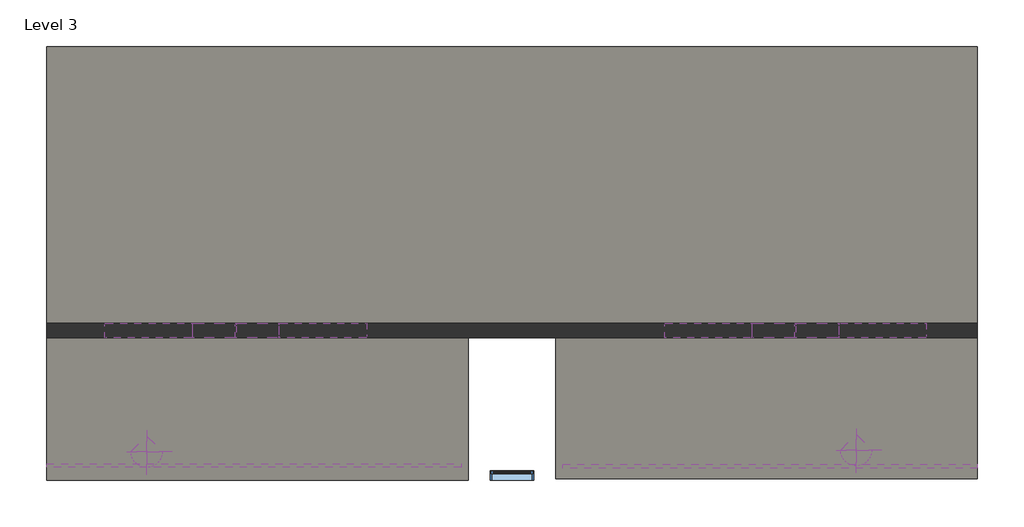
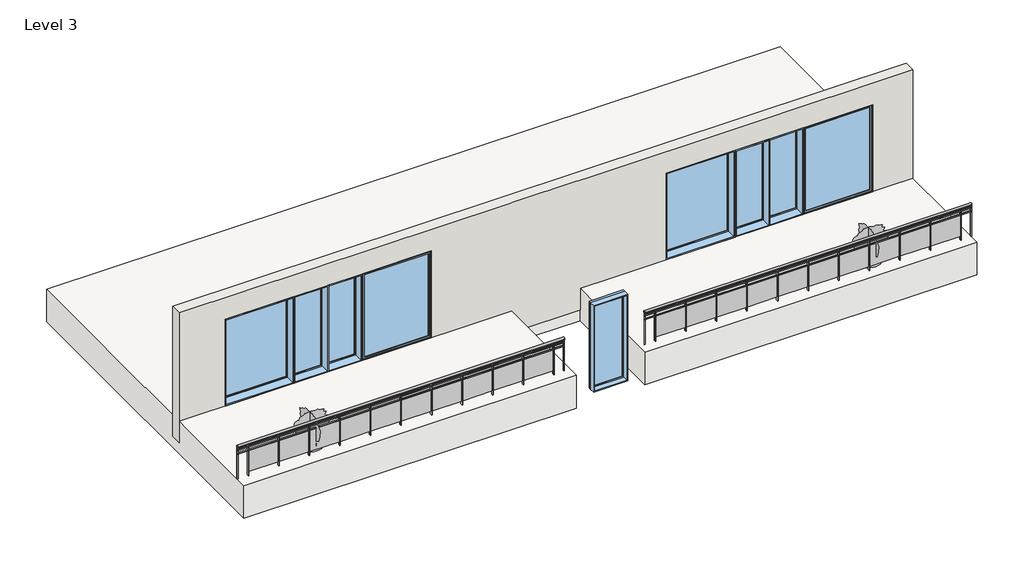
# One storey: 9 windows, 2 geographic elements, 2 railings, 1 slab, 1 wall.
"""IFC4 building model written with IfcOpenShell, lengths in millimetres."""

from ifc_helpers import new_model, si_unit, point, frame, origin, place, context, project, spatial, polyline, ellipse_curve, trimmed, outline, extrude, faceted_brep, transform, mapped, element, save
from ifc_brep_helpers import plane_surface, extruded_surface, advanced_brep
from components import geographic_element_e27c54a3, window_a209d960, window_307ff736, window_1de08d8e, window_9610881e

model = new_model("IFC4")

# Units and contexts
model_context = context("Model", 3, world=origin())
ifc_project = project(units=[si_unit("LENGTHUNIT", "METRE", prefix="MILLI")], contexts=[model_context])

# Site, building, storey
site = spatial("IfcSite", under=ifc_project)
building = spatial("IfcBuilding", under=site)
storey = spatial("IfcBuildingStorey", under=building, Name="Level 3", Elevation=6096.0)

# Geographic elements
placement = place(None, origin())
geographic_element_shape = geographic_element_e27c54a3(model_context)
element("IfcGeographicElement", 1, ObjectType="RPC Shrub : Cedar Shrub 3'-0\"", at=placement, inside=storey, context=model_context, shape_type="MappedRepresentation", body=[
    mapped(geographic_element_shape, transform((-717.5856066, 3526.7740855, 7651.75), x_axis=(1.0, 0.0, 0.0), y_axis=(0.0, 1.0, 0.0), z_axis=(0.0, 0.0, 1.0))),
])
element("IfcGeographicElement", 2, ObjectType="RPC Shrub : Cedar Shrub 3'-0\"", at=placement, inside=storey, context=model_context, shape_type="MappedRepresentation", body=[
    mapped(geographic_element_shape, transform((-15595.2031131, 3490.853061, 7702.55), x_axis=(1.0, 0.0, 0.0), y_axis=(0.0, 1.0, 0.0), z_axis=(0.0, 0.0, 1.0))),
])

# Railings
element("IfcRailing", 3, ObjectType="Glass Panel - Bottom Fill", at=placement, inside=storey, context=model_context, shape_type="SolidModel", body=[
    advanced_brep(
    [(-17688.8338476, 3238.7223265, 8534.4), (-17688.8338476, 3162.5223265, 8534.4), (-9002.0338476, 3238.7223265, 8534.4), (-9002.0338476, 3162.5223265, 8534.4)],
    [
        (0, 1, ellipse_curve(frame((-17688.8338476, 3200.6223265, 8534.4), z_axis=(-1.0, 0.0, 0.0), x_axis=(0.0, -1.0, 0.0)), 38.1, 28.575)),
        (1, 0, ellipse_curve(frame((-17688.8338476, 3200.6223265, 8534.4), z_axis=(-1.0, 0.0, 0.0), x_axis=(0.0, -1.0, 0.0)), 38.1, 28.575)),
        (2, 3, ellipse_curve(frame((-9002.0338476, 3200.6223265, 8534.4), z_axis=(1.0, 0.0, 0.0), x_axis=(0.0, -1.0, 0.0)), 38.1, 28.575)),
        (3, 2, ellipse_curve(frame((-9002.0338476, 3200.6223265, 8534.4), z_axis=(1.0, 0.0, 0.0), x_axis=(0.0, -1.0, 0.0)), 38.1, 28.575)),
        (0, 2),
        (3, 1),
    ],
    [
        plane_surface(frame((-17688.8338476, 3200.6223265, 8534.4), z_axis=(-1.0, 0.0, 0.0), x_axis=(0.0, 1.0, 0.0))),
        plane_surface(frame((-9002.0338476, 3200.6223265, 8534.4), z_axis=(1.0, 0.0, 0.0), x_axis=(0.0, 1.0, 0.0))),
        extruded_surface(trimmed(ellipse_curve(frame((-9002.0338476, 3200.6223265, 8534.4), z_axis=(-1.0, 0.0, 0.0), x_axis=(0.0, -1.0, 0.0)), 38.1, 28.575), [point((-9002.0338476, 3238.7223265, 8534.4))], [point((-9002.0338476, 3162.5223265, 8534.4))], True, "CARTESIAN"), (-8686.8, 0.0, 0.0), 8686.8),
        extruded_surface(trimmed(ellipse_curve(frame((-9002.0338476, 3200.6223265, 8534.4), z_axis=(-1.0, 0.0, 0.0), x_axis=(0.0, -1.0, 0.0)), 38.1, 28.575), [point((-9002.0338476, 3162.5223265, 8534.4))], [point((-9002.0338476, 3238.7223265, 8534.4))], True, "CARTESIAN"), (-8686.8, 0.0, 0.0), 8686.8),
    ],
    [
        (0, [[1, 2]]),
        (1, [[3, 4]]),
        (2, [[-1, 5, -4, 6]]),
        (3, [[-2, -6, -3, -5]]),
    ],
),
    extrude(outline(polyline([(-17688.8338476, 3187.9223265), (-17688.8338476, 3213.3223265), (-9002.0338476, 3213.3223265), (-9002.0338476, 3187.9223265), (-17688.8338476, 3187.9223265)])), frame((0.0, 0.0, 8420.1), z_axis=(0.0, 0.0, 1.0), x_axis=(1.0, 0.0, 0.0)), (0.0, 0.0, 1.0), 25.4),
    extrude(outline(polyline([(-17688.8338476, 3187.9223265), (-17688.8338476, 3213.3223265), (-9002.0338476, 3213.3223265), (-9002.0338476, 3187.9223265), (-17688.8338476, 3187.9223265)])), frame((0.0, 0.0, 8318.5), z_axis=(0.0, 0.0, 1.0), x_axis=(1.0, 0.0, 0.0)), (0.0, 0.0, 1.0), 25.4),
    extrude(outline(polyline([(-9287.7838476, 3175.2223265), (-9287.7838476, 3226.0223265), (-9275.0838476, 3226.0223265), (-9275.0838476, 3175.2223265), (-9287.7838476, 3175.2223265)])), frame((0.0, 0.0, 7620.0), z_axis=(0.0, 0.0, 1.0), x_axis=(1.0, 0.0, 0.0)), (0.0, 0.0, 1.0), 885.6788223),
    extrude(outline(polyline([(-10094.2338476, 3207.1574835), (-9281.4338476, 3207.1574835), (-9281.4338476, 3200.8074835), (-10094.2338476, 3200.8074835), (-10094.2338476, 3207.1574835)])), frame((0.0, 0.0, 7721.6), z_axis=(0.0, 0.0, 1.0), x_axis=(1.0, 0.0, 0.0)), (0.0, 0.0, 1.0), 596.9),
    extrude(outline(polyline([(-10100.5838476, 3175.2223265), (-10100.5838476, 3226.0223265), (-10087.8838476, 3226.0223265), (-10087.8838476, 3175.2223265), (-10100.5838476, 3175.2223265)])), frame((0.0, 0.0, 7620.0), z_axis=(0.0, 0.0, 1.0), x_axis=(1.0, 0.0, 0.0)), (0.0, 0.0, 1.0), 885.6788223),
    extrude(outline(polyline([(-10907.0338476, 3207.1574835), (-10094.2338476, 3207.1574835), (-10094.2338476, 3200.8074835), (-10907.0338476, 3200.8074835), (-10907.0338476, 3207.1574835)])), frame((0.0, 0.0, 7721.6), z_axis=(0.0, 0.0, 1.0), x_axis=(1.0, 0.0, 0.0)), (0.0, 0.0, 1.0), 596.9),
    extrude(outline(polyline([(-10913.3838476, 3175.2223265), (-10913.3838476, 3226.0223265), (-10900.6838476, 3226.0223265), (-10900.6838476, 3175.2223265), (-10913.3838476, 3175.2223265)])), frame((0.0, 0.0, 7620.0), z_axis=(0.0, 0.0, 1.0), x_axis=(1.0, 0.0, 0.0)), (0.0, 0.0, 1.0), 885.6788223),
    extrude(outline(polyline([(-11719.8338476, 3207.1574835), (-10907.0338476, 3207.1574835), (-10907.0338476, 3200.8074835), (-11719.8338476, 3200.8074835), (-11719.8338476, 3207.1574835)])), frame((0.0, 0.0, 7721.6), z_axis=(0.0, 0.0, 1.0), x_axis=(1.0, 0.0, 0.0)), (0.0, 0.0, 1.0), 596.9),
    extrude(outline(polyline([(-11726.1838476, 3175.2223265), (-11726.1838476, 3226.0223265), (-11713.4838476, 3226.0223265), (-11713.4838476, 3175.2223265), (-11726.1838476, 3175.2223265)])), frame((0.0, 0.0, 7620.0), z_axis=(0.0, 0.0, 1.0), x_axis=(1.0, 0.0, 0.0)), (0.0, 0.0, 1.0), 885.6788223),
    extrude(outline(polyline([(-12532.6338476, 3207.1574835), (-11719.8338476, 3207.1574835), (-11719.8338476, 3200.8074835), (-12532.6338476, 3200.8074835), (-12532.6338476, 3207.1574835)])), frame((0.0, 0.0, 7721.6), z_axis=(0.0, 0.0, 1.0), x_axis=(1.0, 0.0, 0.0)), (0.0, 0.0, 1.0), 596.9),
    extrude(outline(polyline([(-12538.9838476, 3175.2223265), (-12538.9838476, 3226.0223265), (-12526.2838476, 3226.0223265), (-12526.2838476, 3175.2223265), (-12538.9838476, 3175.2223265)])), frame((0.0, 0.0, 7620.0), z_axis=(0.0, 0.0, 1.0), x_axis=(1.0, 0.0, 0.0)), (0.0, 0.0, 1.0), 885.6788223),
    extrude(outline(polyline([(-13345.4338476, 3207.1574835), (-12532.6338476, 3207.1574835), (-12532.6338476, 3200.8074835), (-13345.4338476, 3200.8074835), (-13345.4338476, 3207.1574835)])), frame((0.0, 0.0, 7721.6), z_axis=(0.0, 0.0, 1.0), x_axis=(1.0, 0.0, 0.0)), (0.0, 0.0, 1.0), 596.9),
    extrude(outline(polyline([(-13351.7838476, 3175.2223265), (-13351.7838476, 3226.0223265), (-13339.0838476, 3226.0223265), (-13339.0838476, 3175.2223265), (-13351.7838476, 3175.2223265)])), frame((0.0, 0.0, 7620.0), z_axis=(0.0, 0.0, 1.0), x_axis=(1.0, 0.0, 0.0)), (0.0, 0.0, 1.0), 885.6788223),
    extrude(outline(polyline([(-14158.2338476, 3207.1574835), (-13345.4338476, 3207.1574835), (-13345.4338476, 3200.8074835), (-14158.2338476, 3200.8074835), (-14158.2338476, 3207.1574835)])), frame((0.0, 0.0, 7721.6), z_axis=(0.0, 0.0, 1.0), x_axis=(1.0, 0.0, 0.0)), (0.0, 0.0, 1.0), 596.9),
    extrude(outline(polyline([(-14164.5838476, 3175.2223265), (-14164.5838476, 3226.0223265), (-14151.8838476, 3226.0223265), (-14151.8838476, 3175.2223265), (-14164.5838476, 3175.2223265)])), frame((0.0, 0.0, 7620.0), z_axis=(0.0, 0.0, 1.0), x_axis=(1.0, 0.0, 0.0)), (0.0, 0.0, 1.0), 885.6788223),
    extrude(outline(polyline([(-14971.0338476, 3207.1574835), (-14158.2338476, 3207.1574835), (-14158.2338476, 3200.8074835), (-14971.0338476, 3200.8074835), (-14971.0338476, 3207.1574835)])), frame((0.0, 0.0, 7721.6), z_axis=(0.0, 0.0, 1.0), x_axis=(1.0, 0.0, 0.0)), (0.0, 0.0, 1.0), 596.9),
    extrude(outline(polyline([(-14977.3838476, 3175.2223265), (-14977.3838476, 3226.0223265), (-14964.6838476, 3226.0223265), (-14964.6838476, 3175.2223265), (-14977.3838476, 3175.2223265)])), frame((0.0, 0.0, 7620.0), z_axis=(0.0, 0.0, 1.0), x_axis=(1.0, 0.0, 0.0)), (0.0, 0.0, 1.0), 885.6788223),
    extrude(outline(polyline([(-15783.8338476, 3207.1574835), (-14971.0338476, 3207.1574835), (-14971.0338476, 3200.8074835), (-15783.8338476, 3200.8074835), (-15783.8338476, 3207.1574835)])), frame((0.0, 0.0, 7721.6), z_axis=(0.0, 0.0, 1.0), x_axis=(1.0, 0.0, 0.0)), (0.0, 0.0, 1.0), 596.9),
    extrude(outline(polyline([(-15790.1838476, 3175.2223265), (-15790.1838476, 3226.0223265), (-15777.4838476, 3226.0223265), (-15777.4838476, 3175.2223265), (-15790.1838476, 3175.2223265)])), frame((0.0, 0.0, 7620.0), z_axis=(0.0, 0.0, 1.0), x_axis=(1.0, 0.0, 0.0)), (0.0, 0.0, 1.0), 885.6788223),
    extrude(outline(polyline([(-16596.6338476, 3207.1574835), (-15783.8338476, 3207.1574835), (-15783.8338476, 3200.8074835), (-16596.6338476, 3200.8074835), (-16596.6338476, 3207.1574835)])), frame((0.0, 0.0, 7721.6), z_axis=(0.0, 0.0, 1.0), x_axis=(1.0, 0.0, 0.0)), (0.0, 0.0, 1.0), 596.9),
    extrude(outline(polyline([(-16602.9838476, 3175.2223265), (-16602.9838476, 3226.0223265), (-16590.2838476, 3226.0223265), (-16590.2838476, 3175.2223265), (-16602.9838476, 3175.2223265)])), frame((0.0, 0.0, 7620.0), z_axis=(0.0, 0.0, 1.0), x_axis=(1.0, 0.0, 0.0)), (0.0, 0.0, 1.0), 885.6788223),
    extrude(outline(polyline([(-17409.4338476, 3207.1574835), (-16596.6338476, 3207.1574835), (-16596.6338476, 3200.8074835), (-17409.4338476, 3200.8074835), (-17409.4338476, 3207.1574835)])), frame((0.0, 0.0, 7721.6), z_axis=(0.0, 0.0, 1.0), x_axis=(1.0, 0.0, 0.0)), (0.0, 0.0, 1.0), 596.9),
    extrude(outline(polyline([(-17415.7838476, 3175.2223265), (-17415.7838476, 3226.0223265), (-17403.0838476, 3226.0223265), (-17403.0838476, 3175.2223265), (-17415.7838476, 3175.2223265)])), frame((0.0, 0.0, 7620.0), z_axis=(0.0, 0.0, 1.0), x_axis=(1.0, 0.0, 0.0)), (0.0, 0.0, 1.0), 885.6788223),
    extrude(outline(polyline([(-9014.7338476, 3191.0973265), (-9014.7338476, 3210.1473265), (-8995.6838476, 3210.1473265), (-8995.6838476, 3191.0973265), (-9014.7338476, 3191.0973265)])), frame((0.0, 0.0, 7620.0), z_axis=(0.0, 0.0, 1.0), x_axis=(1.0, 0.0, 0.0)), (0.0, 0.0, 1.0), 885.6788223),
    extrude(outline(polyline([(-17695.1838476, 3191.0973265), (-17695.1838476, 3210.1473265), (-17676.1338476, 3210.1473265), (-17676.1338476, 3191.0973265), (-17695.1838476, 3191.0973265)])), frame((0.0, 0.0, 7620.0), z_axis=(0.0, 0.0, 1.0), x_axis=(1.0, 0.0, 0.0)), (0.0, 0.0, 1.0), 885.6788223),
])
element("IfcRailing", 4, ObjectType="Glass Panel - Bottom Fill", at=placement, inside=storey, context=model_context, shape_type="SolidModel", body=[
    advanced_brep(
    [(-6868.4338476, 3226.0223265, 8534.4), (-6868.4338476, 3149.8223265, 8534.4), (1818.3661524, 3226.0223265, 8534.4), (1818.3661524, 3149.8223265, 8534.4)],
    [
        (0, 1, ellipse_curve(frame((-6868.4338476, 3187.9223265, 8534.4), z_axis=(-1.0, 0.0, 0.0), x_axis=(0.0, -1.0, 0.0)), 38.1, 28.575)),
        (1, 0, ellipse_curve(frame((-6868.4338476, 3187.9223265, 8534.4), z_axis=(-1.0, 0.0, 0.0), x_axis=(0.0, -1.0, 0.0)), 38.1, 28.575)),
        (2, 3, ellipse_curve(frame((1818.3661524, 3187.9223265, 8534.4), z_axis=(1.0, 0.0, 0.0), x_axis=(0.0, -1.0, 0.0)), 38.1, 28.575)),
        (3, 2, ellipse_curve(frame((1818.3661524, 3187.9223265, 8534.4), z_axis=(1.0, 0.0, 0.0), x_axis=(0.0, -1.0, 0.0)), 38.1, 28.575)),
        (0, 2),
        (3, 1),
    ],
    [
        plane_surface(frame((-6868.4338476, 3187.9223265, 8534.4), z_axis=(-1.0, 0.0, 0.0), x_axis=(0.0, 1.0, 0.0))),
        plane_surface(frame((1818.3661524, 3187.9223265, 8534.4), z_axis=(1.0, 0.0, 0.0), x_axis=(0.0, 1.0, 0.0))),
        extruded_surface(trimmed(ellipse_curve(frame((1818.3661524, 3187.9223265, 8534.4), z_axis=(-1.0, 0.0, 0.0), x_axis=(0.0, -1.0, 0.0)), 38.1, 28.575), [point((1818.3661524, 3226.0223265, 8534.4))], [point((1818.3661524, 3149.8223265, 8534.4))], True, "CARTESIAN"), (-8686.8, 0.0, 0.0), 8686.8),
        extruded_surface(trimmed(ellipse_curve(frame((1818.3661524, 3187.9223265, 8534.4), z_axis=(-1.0, 0.0, 0.0), x_axis=(0.0, -1.0, 0.0)), 38.1, 28.575), [point((1818.3661524, 3149.8223265, 8534.4))], [point((1818.3661524, 3226.0223265, 8534.4))], True, "CARTESIAN"), (-8686.8, 0.0, 0.0), 8686.8),
    ],
    [
        (0, [[1, 2]]),
        (1, [[3, 4]]),
        (2, [[-1, 5, -4, 6]]),
        (3, [[-2, -6, -3, -5]]),
    ],
),
    extrude(outline(polyline([(-6868.4338476, 3175.2223265), (-6868.4338476, 3200.6223265), (1818.3661524, 3200.6223265), (1818.3661524, 3175.2223265), (-6868.4338476, 3175.2223265)])), frame((0.0, 0.0, 8420.1), z_axis=(0.0, 0.0, 1.0), x_axis=(1.0, 0.0, 0.0)), (0.0, 0.0, 1.0), 25.4),
    extrude(outline(polyline([(-6868.4338476, 3175.2223265), (-6868.4338476, 3200.6223265), (1818.3661524, 3200.6223265), (1818.3661524, 3175.2223265), (-6868.4338476, 3175.2223265)])), frame((0.0, 0.0, 8318.5), z_axis=(0.0, 0.0, 1.0), x_axis=(1.0, 0.0, 0.0)), (0.0, 0.0, 1.0), 25.4),
    extrude(outline(polyline([(1532.6161524, 3162.5223265), (1532.6161524, 3213.3223265), (1545.3161524, 3213.3223265), (1545.3161524, 3162.5223265), (1532.6161524, 3162.5223265)])), frame((0.0, 0.0, 7620.0), z_axis=(0.0, 0.0, 1.0), x_axis=(1.0, 0.0, 0.0)), (0.0, 0.0, 1.0), 885.6788223),
    extrude(outline(polyline([(726.1661524, 3194.4574835), (1538.9661524, 3194.4574835), (1538.9661524, 3188.1074835), (726.1661524, 3188.1074835), (726.1661524, 3194.4574835)])), frame((0.0, 0.0, 7721.6), z_axis=(0.0, 0.0, 1.0), x_axis=(1.0, 0.0, 0.0)), (0.0, 0.0, 1.0), 596.9),
    extrude(outline(polyline([(719.8161524, 3162.5223265), (719.8161524, 3213.3223265), (732.5161524, 3213.3223265), (732.5161524, 3162.5223265), (719.8161524, 3162.5223265)])), frame((0.0, 0.0, 7620.0), z_axis=(0.0, 0.0, 1.0), x_axis=(1.0, 0.0, 0.0)), (0.0, 0.0, 1.0), 885.6788223),
    extrude(outline(polyline([(-86.6338476, 3194.4574835), (726.1661524, 3194.4574835), (726.1661524, 3188.1074835), (-86.6338476, 3188.1074835), (-86.6338476, 3194.4574835)])), frame((0.0, 0.0, 7721.6), z_axis=(0.0, 0.0, 1.0), x_axis=(1.0, 0.0, 0.0)), (0.0, 0.0, 1.0), 596.9),
    extrude(outline(polyline([(-92.9838476, 3162.5223265), (-92.9838476, 3213.3223265), (-80.2838476, 3213.3223265), (-80.2838476, 3162.5223265), (-92.9838476, 3162.5223265)])), frame((0.0, 0.0, 7620.0), z_axis=(0.0, 0.0, 1.0), x_axis=(1.0, 0.0, 0.0)), (0.0, 0.0, 1.0), 885.6788223),
    extrude(outline(polyline([(-899.4338476, 3194.4574835), (-86.6338476, 3194.4574835), (-86.6338476, 3188.1074835), (-899.4338476, 3188.1074835), (-899.4338476, 3194.4574835)])), frame((0.0, 0.0, 7721.6), z_axis=(0.0, 0.0, 1.0), x_axis=(1.0, 0.0, 0.0)), (0.0, 0.0, 1.0), 596.9),
    extrude(outline(polyline([(-905.7838476, 3162.5223265), (-905.7838476, 3213.3223265), (-893.0838476, 3213.3223265), (-893.0838476, 3162.5223265), (-905.7838476, 3162.5223265)])), frame((0.0, 0.0, 7620.0), z_axis=(0.0, 0.0, 1.0), x_axis=(1.0, 0.0, 0.0)), (0.0, 0.0, 1.0), 885.6788223),
    extrude(outline(polyline([(-1712.2338476, 3194.4574835), (-899.4338476, 3194.4574835), (-899.4338476, 3188.1074835), (-1712.2338476, 3188.1074835), (-1712.2338476, 3194.4574835)])), frame((0.0, 0.0, 7721.6), z_axis=(0.0, 0.0, 1.0), x_axis=(1.0, 0.0, 0.0)), (0.0, 0.0, 1.0), 596.9),
    extrude(outline(polyline([(-1718.5838476, 3162.5223265), (-1718.5838476, 3213.3223265), (-1705.8838476, 3213.3223265), (-1705.8838476, 3162.5223265), (-1718.5838476, 3162.5223265)])), frame((0.0, 0.0, 7620.0), z_axis=(0.0, 0.0, 1.0), x_axis=(1.0, 0.0, 0.0)), (0.0, 0.0, 1.0), 885.6788223),
    extrude(outline(polyline([(-2525.0338476, 3194.4574835), (-1712.2338476, 3194.4574835), (-1712.2338476, 3188.1074835), (-2525.0338476, 3188.1074835), (-2525.0338476, 3194.4574835)])), frame((0.0, 0.0, 7721.6), z_axis=(0.0, 0.0, 1.0), x_axis=(1.0, 0.0, 0.0)), (0.0, 0.0, 1.0), 596.9),
    extrude(outline(polyline([(-2531.3838476, 3162.5223265), (-2531.3838476, 3213.3223265), (-2518.6838476, 3213.3223265), (-2518.6838476, 3162.5223265), (-2531.3838476, 3162.5223265)])), frame((0.0, 0.0, 7620.0), z_axis=(0.0, 0.0, 1.0), x_axis=(1.0, 0.0, 0.0)), (0.0, 0.0, 1.0), 885.6788223),
    extrude(outline(polyline([(-3337.8338476, 3194.4574835), (-2525.0338476, 3194.4574835), (-2525.0338476, 3188.1074835), (-3337.8338476, 3188.1074835), (-3337.8338476, 3194.4574835)])), frame((0.0, 0.0, 7721.6), z_axis=(0.0, 0.0, 1.0), x_axis=(1.0, 0.0, 0.0)), (0.0, 0.0, 1.0), 596.9),
    extrude(outline(polyline([(-3344.1838476, 3162.5223265), (-3344.1838476, 3213.3223265), (-3331.4838476, 3213.3223265), (-3331.4838476, 3162.5223265), (-3344.1838476, 3162.5223265)])), frame((0.0, 0.0, 7620.0), z_axis=(0.0, 0.0, 1.0), x_axis=(1.0, 0.0, 0.0)), (0.0, 0.0, 1.0), 885.6788223),
    extrude(outline(polyline([(-4150.6338476, 3194.4574835), (-3337.8338476, 3194.4574835), (-3337.8338476, 3188.1074835), (-4150.6338476, 3188.1074835), (-4150.6338476, 3194.4574835)])), frame((0.0, 0.0, 7721.6), z_axis=(0.0, 0.0, 1.0), x_axis=(1.0, 0.0, 0.0)), (0.0, 0.0, 1.0), 596.9),
    extrude(outline(polyline([(-4156.9838476, 3162.5223265), (-4156.9838476, 3213.3223265), (-4144.2838476, 3213.3223265), (-4144.2838476, 3162.5223265), (-4156.9838476, 3162.5223265)])), frame((0.0, 0.0, 7620.0), z_axis=(0.0, 0.0, 1.0), x_axis=(1.0, 0.0, 0.0)), (0.0, 0.0, 1.0), 885.6788223),
    extrude(outline(polyline([(-4963.4338476, 3194.4574835), (-4150.6338476, 3194.4574835), (-4150.6338476, 3188.1074835), (-4963.4338476, 3188.1074835), (-4963.4338476, 3194.4574835)])), frame((0.0, 0.0, 7721.6), z_axis=(0.0, 0.0, 1.0), x_axis=(1.0, 0.0, 0.0)), (0.0, 0.0, 1.0), 596.9),
    extrude(outline(polyline([(-4969.7838476, 3162.5223265), (-4969.7838476, 3213.3223265), (-4957.0838476, 3213.3223265), (-4957.0838476, 3162.5223265), (-4969.7838476, 3162.5223265)])), frame((0.0, 0.0, 7620.0), z_axis=(0.0, 0.0, 1.0), x_axis=(1.0, 0.0, 0.0)), (0.0, 0.0, 1.0), 885.6788223),
    extrude(outline(polyline([(-5776.2338476, 3194.4574835), (-4963.4338476, 3194.4574835), (-4963.4338476, 3188.1074835), (-5776.2338476, 3188.1074835), (-5776.2338476, 3194.4574835)])), frame((0.0, 0.0, 7721.6), z_axis=(0.0, 0.0, 1.0), x_axis=(1.0, 0.0, 0.0)), (0.0, 0.0, 1.0), 596.9),
    extrude(outline(polyline([(-5782.5838476, 3162.5223265), (-5782.5838476, 3213.3223265), (-5769.8838476, 3213.3223265), (-5769.8838476, 3162.5223265), (-5782.5838476, 3162.5223265)])), frame((0.0, 0.0, 7620.0), z_axis=(0.0, 0.0, 1.0), x_axis=(1.0, 0.0, 0.0)), (0.0, 0.0, 1.0), 885.6788223),
    extrude(outline(polyline([(-6589.0338476, 3194.4574835), (-5776.2338476, 3194.4574835), (-5776.2338476, 3188.1074835), (-6589.0338476, 3188.1074835), (-6589.0338476, 3194.4574835)])), frame((0.0, 0.0, 7721.6), z_axis=(0.0, 0.0, 1.0), x_axis=(1.0, 0.0, 0.0)), (0.0, 0.0, 1.0), 596.9),
    extrude(outline(polyline([(-6595.3838476, 3162.5223265), (-6595.3838476, 3213.3223265), (-6582.6838476, 3213.3223265), (-6582.6838476, 3162.5223265), (-6595.3838476, 3162.5223265)])), frame((0.0, 0.0, 7620.0), z_axis=(0.0, 0.0, 1.0), x_axis=(1.0, 0.0, 0.0)), (0.0, 0.0, 1.0), 885.6788223),
    extrude(outline(polyline([(1805.6661524, 3178.3973265), (1805.6661524, 3197.4473265), (1824.7161524, 3197.4473265), (1824.7161524, 3178.3973265), (1805.6661524, 3178.3973265)])), frame((0.0, 0.0, 7620.0), z_axis=(0.0, 0.0, 1.0), x_axis=(1.0, 0.0, 0.0)), (0.0, 0.0, 1.0), 885.6788223),
    extrude(outline(polyline([(-6874.7838476, 3178.3973265), (-6874.7838476, 3197.4473265), (-6855.7338476, 3197.4473265), (-6855.7338476, 3178.3973265), (-6874.7838476, 3178.3973265)])), frame((0.0, 0.0, 7620.0), z_axis=(0.0, 0.0, 1.0), x_axis=(1.0, 0.0, 0.0)), (0.0, 0.0, 1.0), 885.6788223),
])

# Slab
element("IfcSlab", 5, ObjectType="Generic - 3'", at=placement, inside=storey, context=model_context, shape_type="SweptSolid", body=[
    extrude(outline(polyline([(1818.3661524, 11989.0223265), (1818.3661524, 2921.2223265), (-7020.8338476, 2921.2223265), (-7020.8338476, 5893.0223265), (-8849.6338476, 5893.0223265), (-8849.6338476, 2895.8223265), (-17688.8338476, 2895.8223265), (-17688.8338476, 11989.0223265), (1818.3661524, 11989.0223265)])), frame((0.0, 0.0, 6705.6), z_axis=(0.0, 0.0, 1.0), x_axis=(1.0, 0.0, 0.0)), (0.0, 0.0, 1.0), 914.4),
])

# Wall
element("IfcWall", 6, ObjectType="Generic - 12\" black", at=placement, inside=storey, context=model_context, shape_type="Brep", body=[
    faceted_brep([(-17688.8338476, 5880.3223265, 7010.4), (1818.3661524, 5880.3223265, 7010.4), (1818.3661524, 5880.3223265, 10668.0), (-6868.4338476, 5880.3223265, 10668.0), (-7173.2338476, 5880.3223265, 10668.0), (-8697.2338476, 5880.3223265, 10668.0), (-9002.0338476, 5880.3223265, 10668.0), (-17688.8338476, 5880.3223265, 10668.0), (751.5661524, 5880.3223265, 10058.4), (751.5661524, 5880.3223265, 7620.0), (-1077.2338476, 5880.3223265, 7620.0), (-1077.2338476, 5880.3223265, 10058.4), (-1086.7588476, 5880.3223265, 10052.683689), (-1086.7588476, 5880.3223265, 7614.283689), (-2896.5088476, 5880.3223265, 7614.283689), (-2896.5088476, 5880.3223265, 10052.683689), (-2906.0338476, 5880.3223265, 10058.4), (-2906.0338476, 5880.3223265, 7620.0), (-4734.8338476, 5880.3223265, 7620.0), (-4734.8338476, 5880.3223265, 10058.4), (-10983.2338476, 5880.3223265, 10058.4), (-10983.2338476, 5880.3223265, 7620.0), (-12812.0338476, 5880.3223265, 7620.0), (-12812.0338476, 5880.3223265, 10058.4), (-14631.3088476, 5880.3223265, 10052.683689), (-12821.5588476, 5880.3223265, 10052.683689), (-12821.5588476, 5880.3223265, 7614.283689), (-14631.3088476, 5880.3223265, 7614.283689), (-14640.8338476, 5880.3223265, 10058.4), (-14640.8338476, 5880.3223265, 7620.0), (-16469.6338476, 5880.3223265, 7620.0), (-16469.6338476, 5880.3223265, 10058.4), (1818.3661524, 6185.1223265, 7010.4), (-17688.8338476, 6185.1223265, 7010.4), (-17688.8338476, 6185.1223265, 10668.0), (1818.3661524, 6185.1223265, 10668.0), (751.5661524, 6185.1223265, 10058.4), (-1077.2338476, 6185.1223265, 10058.4), (-1077.2338476, 6185.1223265, 7620.0), (751.5661524, 6185.1223265, 7620.0), (-1086.7588476, 6185.1223265, 7614.283689), (-1086.7588476, 6185.1223265, 10052.683689), (-2896.5088476, 6185.1223265, 10052.683689), (-2896.5088476, 6185.1223265, 7614.283689), (-2906.0338476, 6185.1223265, 10058.4), (-4734.8338476, 6185.1223265, 10058.4), (-4734.8338476, 6185.1223265, 7620.0), (-2906.0338476, 6185.1223265, 7620.0), (-10983.2338476, 6185.1223265, 10058.4), (-12812.0338476, 6185.1223265, 10058.4), (-12812.0338476, 6185.1223265, 7620.0), (-10983.2338476, 6185.1223265, 7620.0), (-14631.3088476, 6185.1223265, 7614.283689), (-12821.5588476, 6185.1223265, 7614.283689), (-12821.5588476, 6185.1223265, 10052.683689), (-14631.3088476, 6185.1223265, 10052.683689), (-14640.8338476, 6185.1223265, 10058.4), (-16469.6338476, 6185.1223265, 10058.4), (-16469.6338476, 6185.1223265, 7620.0), (-14640.8338476, 6185.1223265, 7620.0)], [[[0, 1, 2, 3, 4, 5, 6, 7], [8, 9, 10, 11], [12, 13, 14, 15], [16, 17, 18, 19], [20, 21, 22, 23], [24, 25, 26, 27], [28, 29, 30, 31]], [[32, 33, 34, 35], [36, 37, 38, 39], [40, 41, 42, 43], [44, 45, 46, 47], [48, 49, 50, 51], [52, 53, 54, 55], [56, 57, 58, 59]], [[1, 0, 33, 32]], [[7, 6, 5, 4, 3, 2, 35, 34]], [[0, 7, 34, 33]], [[2, 1, 32, 35]], [[9, 8, 36, 39]], [[10, 9, 39, 38]], [[11, 10, 38, 37]], [[8, 11, 37, 36]], [[13, 12, 41, 40]], [[13, 40, 43, 14]], [[41, 12, 15, 42]], [[14, 43, 42, 15]], [[17, 16, 44, 47]], [[18, 17, 47, 46]], [[19, 18, 46, 45]], [[16, 19, 45, 44]], [[21, 20, 48, 51]], [[22, 21, 51, 50]], [[23, 22, 50, 49]], [[20, 23, 49, 48]], [[26, 25, 54, 53]], [[26, 53, 52, 27]], [[54, 25, 24, 55]], [[27, 52, 55, 24]], [[29, 28, 56, 59]], [[30, 29, 59, 58]], [[31, 30, 58, 57]], [[28, 31, 57, 56]]]),
])

# Windows
window_shape = window_a209d960(model_context)
element("IfcWindow", 7, ObjectType="Fixed : 36\" x 96\"", at=placement, inside=storey, context=model_context, shape_type="MappedRepresentation", body=[
    mapped(window_shape, transform((-2401.2088476, 6032.7223265, 7309.483689), x_axis=(1.0, 0.0, 0.0), y_axis=(0.0, 1.0, 0.0), z_axis=(0.0, 0.0, 1.0))),
])
element("IfcWindow", 8, ObjectType="Fixed : 36\" x 96\"", at=placement, inside=storey, context=model_context, shape_type="MappedRepresentation", body=[
    mapped(window_shape, transform((-1505.8588476, 6032.7223265, 7309.483689), x_axis=(1.0, 0.0, 0.0), y_axis=(0.0, 1.0, 0.0), z_axis=(0.0, 0.0, 1.0))),
])
element("IfcWindow", 9, ObjectType="Fixed : 36\" x 96\"", at=placement, inside=storey, context=model_context, shape_type="MappedRepresentation", body=[
    mapped(window_shape, transform((-14136.0088476, 6032.7223265, 7309.483689), x_axis=(1.0, 0.0, 0.0), y_axis=(0.0, 1.0, 0.0), z_axis=(0.0, 0.0, 1.0))),
])
element("IfcWindow", 10, ObjectType="Fixed : 36\" x 96\"", at=placement, inside=storey, context=model_context, shape_type="MappedRepresentation", body=[
    mapped(window_shape, transform((-13240.6588476, 6032.7223265, 7309.483689), x_axis=(1.0, 0.0, 0.0), y_axis=(0.0, 1.0, 0.0), z_axis=(0.0, 0.0, 1.0))),
])
window_2_shape = window_307ff736(model_context)
element("IfcWindow", 11, ObjectType="Fixed : 36\" x 96\"", at=placement, inside=storey, context=model_context, shape_type="MappedRepresentation", body=[
    mapped(window_2_shape, transform((-7897.1338476, 2997.4223265, 6683.6097194), x_axis=(1.0, 0.0, 0.0), y_axis=(0.0, 1.0, 0.0), z_axis=(0.0, 0.0, 1.0))),
])
window_3_shape = window_1de08d8e(model_context)
element("IfcWindow", 12, ObjectType="Fixed : 72\" x 96\"", at=placement, inside=storey, context=model_context, shape_type="MappedRepresentation", body=[
    mapped(window_3_shape, transform((-3782.3338476, 6032.7223265, 7315.2), x_axis=(1.0, 0.0, 0.0), y_axis=(0.0, 1.0, 0.0), z_axis=(0.0, 0.0, 1.0))),
])
element("IfcWindow", 13, ObjectType="Fixed : 72\" x 96\"", at=placement, inside=storey, context=model_context, shape_type="MappedRepresentation", body=[
    mapped(window_3_shape, transform((-15517.1338476, 6032.7223265, 7315.2), x_axis=(1.0, 0.0, 0.0), y_axis=(0.0, 1.0, 0.0), z_axis=(0.0, 0.0, 1.0))),
])
window_4_shape = window_9610881e(model_context)
element("IfcWindow", 14, ObjectType="Fixed : 72\" x 96\"", at=placement, inside=storey, context=model_context, shape_type="MappedRepresentation", body=[
    mapped(window_4_shape, transform((-124.7338476, 6032.7223265, 7315.2), x_axis=(1.0, 0.0, 0.0), y_axis=(0.0, 1.0, 0.0), z_axis=(0.0, 0.0, 1.0))),
])
element("IfcWindow", 15, ObjectType="Fixed : 72\" x 96\"", at=placement, inside=storey, context=model_context, shape_type="MappedRepresentation", body=[
    mapped(window_4_shape, transform((-11859.5338476, 6032.7223265, 7315.2), x_axis=(1.0, 0.0, 0.0), y_axis=(0.0, 1.0, 0.0), z_axis=(0.0, 0.0, 1.0))),
])

save(model, "model.ifc")

# Revit data of these elements
# Type "RPC Shrub : Cedar Shrub 3'-0\""
#   Type Comments = "Cedar Shrub"
#   built-in parameter 1005198 = "{2, 15},{39, RPC-16-FUMD-ULXX-U7X6-J000-ST1L-LVER-AU},{1, 0},{1, 0},{2, 13},{1, 8},{5, Color},{1, 0},{1, 0},{3, 0.8},{3, 0.8},{3, 0.8},{1, 8},{7, BBoxMin},{1, 0},{1, 0},{1, 0},{1, 0},{1, 0},{1, 8},{7, BBoxMax},{1, 0},{1, 0},{1, 0},{1, 0},{1, 0},{2, 11},{9, RPCTypeId},{1, 0},{1, 0},{39, RPC-16-FUMD-ULXX-U7X6-J000-ST1L-LVER-AU},{1, 6},{14, RPCPlantHeight},{1, 0},{1, 0},{1, 3},{2, 11},{7, keyword},{1, 0},{1, 0},{35, :RPCs:Shrubs [General]:Geometry:RPC},{2, 11},{8, category},{1, 0},{1, 0},{16, Shrubs [General]},{2, 11},{12, LocalizedUID},{1, 0},{1, 0},{11, Cedar Shrub},{2, 14},{6, Height},{1, 0},{1, 0},{1, 3},{1, 2},{16, Cast Reflections},{1, 0},{1, 0},{1, 0},{1, 2},{12, Cast Shadows},{1, 0},{1, 0},{1, 1},{1, 2},{9, Lock View},{1, 0},{1, 0},{1, 0},{1, 4},{5, ViewC},{1, 0},{1, 0},{1, 0},{21, assetlibrary_base.fbx},{1, 5},"
#   built-in parameter 1005195 = "RPC-16-FUMD-ULXX-U7X6-J000-ST1L-LVER-AU"
#   Assembly Code = "G2050500"
#   Height = 3' - 0"
#   Default Elevation = 0
# Type "Glass Panel - Bottom Fill"
#   Assembly Code = "C2010400"
#   built-in parameter 1008612 = 0.0416667 (stored number, unit not read)
#   built-in parameter 1008611 = 0.0416667 (stored number, unit not read)
#   built-in parameter 1008609 = 0.333333 (stored number, unit not read)
#   built-in parameter 1008604 = 0.166667 (stored number, unit not read)
#   built-in parameter 1008603 = 0.166667 (stored number, unit not read)
#   Railing Height = 3' - 0"
#   built-in parameter 1008630 = 2
#   built-in parameter 1008610 = 2
#   built-in parameter 1008618 = Baluster - Square : 3/4"
# Type "Generic - 3'"
#   Assembly Code = "B1010"
#   Function = 0
#   Layers, outside or top first: 3' - 0" "Concrete Masonry Units" (function 1)
# Type "Generic - 12\" black"
#   Assembly Code = "B2010"
#   Layers, outside or top first: 1' - 0" "Parking Stripe" (function 1)
# Type "Fixed : 36\" x 96\""
#   Type Mark = "9"
#   Construction Type Id = "GSP4R"
#   Assembly Code = "B2020100"
#   Analytic Construction = "1/8 in Pilkington single glazing"
#   Visual Light Transmittance = 0.9
#   Solar Heat Gain Coefficient = 0.78
#   Heat Transfer Coefficient (U) = 0.6496 BTU/(h·ft²·°F)
#   Height = 8' - 0"
#   Default Sill Height = 1' - 0"
#   Width = 3' - 0"
#   Window Inset = 0' - 0 3/4"
#   Define Thermal Properties by = 1
#   Glass Pane Material = Glass
#   Sash Material = Iron, Ductile
#   Wall Closure = (empty or 0)
# Type "Fixed : 72\" x 96\""
#   Type Mark = "11"
#   Construction Type Id = "GSP4R"
#   Assembly Code = "B2020100"
#   Analytic Construction = "1/8 in Pilkington single glazing"
#   Visual Light Transmittance = 0.9
#   Solar Heat Gain Coefficient = 0.78
#   Heat Transfer Coefficient (U) = 0.6496 BTU/(h·ft²·°F)
#   Height = 8' - 0"
#   Default Sill Height = 1' - 0"
#   Width = 6' - 0"
#   Window Inset = 0' - 0 3/4"
#   Define Thermal Properties by = 1
#   Glass Pane Material = Glass
#   Sash Material = Iron, Ductile
#   Wall Closure = (empty or 0)
# Elements 1, 2 (IfcGeographicElement, "RPC Shrub : Cedar Shrub 3'-0\"")
#   Phase Created = New Construction
# Elements 3, 4 (IfcRailing, "Glass Panel - Bottom Fill")
#   built-in parameter 1008621 = 5 (stored number, unit not read)
#   Phase Created = New Construction
#   Materials on its faces: "Glass"
# Element 5 (IfcSlab, "Generic - 3'")
#   Height Offset From Level = 5' - 0"
#   Phase Created = New Construction
#   Materials on its faces: "Concrete Masonry Units"
# Element 6 (IfcWall, "Generic - 12\" black")
#   built-in parameter 1001111 = 3' - 0"
#   Top Offset = 0' - 0"
#   Base Offset = 3' - 0"
#   Unconnected Height = 12' - 0"
#   wall height = 12' - 0"
#   Phase Created = New Construction
#   Base Constraint = Level 3
#   Materials on its faces: "Parking Stripe"
# Element 7 (IfcWindow, "Fixed : 36\" x 96\"")
#   Mark = "17"
#   Phase Created = New Construction
#   Materials on its faces: "Iron, Ductile", "Glass"
# Element 8 (IfcWindow, "Fixed : 36\" x 96\"")
#   Mark = "18"
#   Phase Created = New Construction
#   Materials on its faces: "Iron, Ductile", "Glass"
# Element 9 (IfcWindow, "Fixed : 36\" x 96\"")
#   Mark = "21"
#   Phase Created = New Construction
#   Materials on its faces: "Iron, Ductile", "Glass"
# Element 10 (IfcWindow, "Fixed : 36\" x 96\"")
#   Mark = "22"
#   Phase Created = New Construction
#   Materials on its faces: "Iron, Ductile", "Glass"
# Element 11 (IfcWindow, "Fixed : 36\" x 96\"")
#   Mark = "24"
#   Phase Created = New Construction
#   Materials on its faces: "Iron, Ductile", "Glass"
# Element 12 (IfcWindow, "Fixed : 72\" x 96\"")
#   Mark = "16"
#   Phase Created = New Construction
#   Materials on its faces: "Iron, Ductile", "Glass"
# Element 13 (IfcWindow, "Fixed : 72\" x 96\"")
#   Mark = "20"
#   Phase Created = New Construction
#   Materials on its faces: "Iron, Ductile", "Glass"
# Element 14 (IfcWindow, "Fixed : 72\" x 96\"")
#   Mark = "19"
#   Phase Created = New Construction
#   Materials on its faces: "Iron, Ductile", "Glass"
# Element 15 (IfcWindow, "Fixed : 72\" x 96\"")
#   Mark = "23"
#   Phase Created = New Construction
#   Materials on its faces: "Iron, Ductile", "Glass"
# Materials
#   "Concrete Masonry Units": class "Masonry", colour RGB 227 227 227, transparency 0, Description = "Concrete masonry units", Cost = 0
#   "Parking Stripe": class "Paint", colour RGB 250 250 91, transparency 0, Cost = 0
#   "Glass": class "Glass", colour RGB 0 128 192, transparency 0.75, Description = "Soda Lime Glass", Cost = 0
#   "Iron, Ductile": class "Metal", colour RGB 0 0 0, transparency 0, Description = "Ductile cast iron", Cost = 0
